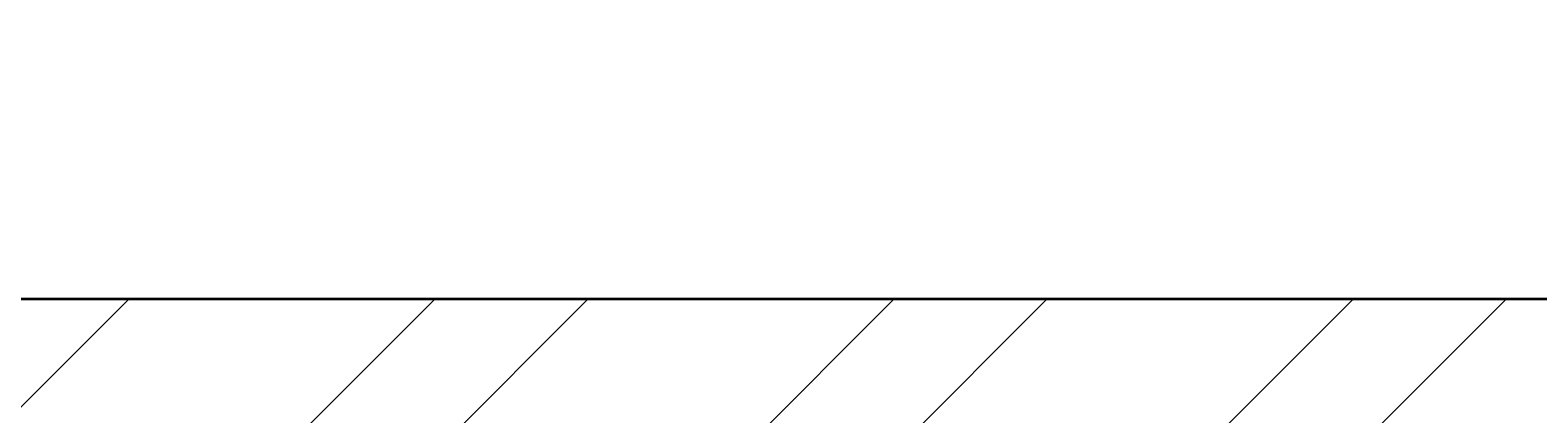
# Model space of a CAD drawing. Units: inches. Extents: x 1962 to 2771, y 1245 to 2660.
# Tile 41 of 114: x 2116 to 2160, y 2030 to 2042. Entities that reach past the tile are written whole.
import ezdxf

# ---------------------------------------------------------------- set-up
doc = ezdxf.new("R2010")
doc.units = ezdxf.units.IN
for name, color, linetype, lineweight in [('A-ANNO-DIMS', 2, 'Continuous', 18), ('A-WALL', 7, 'Continuous', 35), ('A-WALL-PATT', 252, 'Continuous', 13)]:
    doc.layers.add(name, color=color, linetype=linetype, lineweight=lineweight)
doc.styles.get("Standard").update_dxf_attribs({"font": 'arial.ttf'})
doc.dimstyles.get("Standard").update_dxf_attribs({"dimtxt": 0.18, "dimasz": 0.18, "dimexe": 0.18, "dimexo": 0.0625, "dimgap": 0.09, "dimtad": 0, "dimtih": 1, "dimtoh": 1, "dimdec": 4, "dimzin": 0, "dimdsep": 46, "dimtxsty": 'Standard', "dimcen": 0.09, "dimadec": 0, "dimazin": 0, "dimtfac": 1, "dimtdec": 4, "dimtofl": 0, "dimtmove": 0, "dimatfit": 3, "dimfxl": 1, "dimtolj": 1, "dimtzin": 0, "dimarcsym": 0})

# ---------------------------------------------------------------- blocks, each defined once
blk = doc.blocks.new('*D40')
at = {"layer": 'A-ANNO-DIMS', "color": 0, "lineweight": -2, "transparency": 16777216}
for p, q in [((2072.02, 2033.906), (2072.02, 2583.474)), ((2072.2, 2583.294), (2366.02, 2583.294)), ((2660.627, 2583.294), (2366.808, 2583.294)), ((2660.807, 2524.406), (2660.807, 2583.474))]:
    blk.add_line(p, q, dxfattribs=at)
at = {"layer": 'A-ANNO-DIMS', "color": 0, "transparency": 16777216}
for points in [[(2072.2, 2583.324), (2072.2, 2583.264), (2072.02, 2583.294)], [(2660.627, 2583.324), (2660.627, 2583.264), (2660.807, 2583.294)]]:
    blk.add_solid(points, dxfattribs=at)
at = {"layer": 'Defpoints', "color": 0, "transparency": 16777216}
for p in [(2660.807, 2583.294), (2660.807, 2524.344), (2072.02, 2033.844)]:
    blk.add_point(p, dxfattribs=at)
at = {"layer": 'A-ANNO-DIMS', "color": 0, "transparency": 16777216, "insert": (2366.414, 2583.294), "char_height": 0.18, "attachment_point": 5}
blk.add_mtext('\\A1;588.8', dxfattribs=at)

msp = doc.modelspace()

# ---------------------------------------------------------------- hatches: boundary and pattern name
at = {"layer": 'A-WALL-PATT'}
h = msp.add_hatch(dxfattribs=at)
h.set_pattern_fill('ANSI32', color=256)
h.paths.add_polyline_path([(2090.8074, 2467.3437), (2141.6481, 2467.3437), (2141.6481, 2469.5937), (2141.6481, 2471.8437), (2086.3074, 2471.8437), (2086.3074, 2422.5333), (2090.8074, 2422.5333)])
h.paths.add_polyline_path([(2282.7664, 2471.8437), (2204.8982, 2471.8437), (2204.8982, 2467.3437), (2234.8074, 2467.3437), (2234.8074, 2311.3437), (2228.7492, 2311.3437), (2228.7492, 2306.8437), (2234.8074, 2306.8437), (2331.9227, 2306.8437), (2331.9227, 2309.0937), (2331.9227, 2311.3437), (2239.3074, 2311.3437), (2239.3074, 2467.3437), (2282.7664, 2467.3437), (2282.7664, 2469.5937)])
h.paths.add_polyline_path([(2471.4531, 2519.8437), (2552.011, 2519.8437), (2564.3996, 2519.8437), (2564.3996, 2511.1389), (2568.8996, 2511.1389), (2568.8996, 2524.3437), (2466.9531, 2524.3437), (2466.9531, 2471.8437), (2450.0749, 2471.8437), (2446.4672, 2471.8437), (2446.4672, 2467.3437), (2450.0749, 2467.3437), (2475.9988, 2467.3437), (2475.9988, 2469.5937), (2475.9988, 2471.8437), (2471.4531, 2471.8437)])
h.paths.add_polyline_path([(2575.2231, 2469.5937), (2575.2231, 2471.8437), (2568.8996, 2471.8437), (2568.8996, 2487.1389), (2564.3996, 2487.1389), (2564.3996, 2471.8437), (2556.511, 2471.8437), (2499.2904, 2471.8437), (2499.2904, 2467.3437), (2507.8074, 2467.3437), (2507.8074, 2311.3437), (2414.863, 2311.3437), (2414.863, 2306.8437), (2512.3074, 2306.8437), (2517.0114, 2306.8437), (2517.0114, 2309.0937), (2517.0114, 2311.3437), (2512.3074, 2311.3437), (2512.3074, 2467.3437), (2575.2231, 2467.3437)])
h.paths.add_polyline_path([(2660.8074, 2471.8437), (2600.9602, 2471.8437), (2600.9602, 2467.3437), (2656.3074, 2467.3437), (2656.3074, 2432.5704), (2660.8074, 2432.5704)])
h.paths.add_polyline_path([(2660.8074, 2372.5704), (2656.3074, 2372.5704), (2656.3074, 2311.3437), (2600.276, 2311.3437), (2600.276, 2309.0937), (2600.276, 2306.8437), (2656.3074, 2306.8437), (2656.3074, 2296.2593), (2660.8074, 2296.2593)])
h.paths.add_polyline_path([(2572.3074, 2306.8437), (2577.1385, 2306.8437), (2577.1385, 2311.3437), (2551.082, 2311.3437), (2551.082, 2306.8437), (2567.8074, 2306.8437), (2567.8074, 2258.8437), (2540.0574, 2258.8437), (2540.0574, 2256.5937), (2540.0574, 2254.3437), (2567.8074, 2254.3437), (2656.3074, 2254.3437), (2656.3074, 2236.9085), (2660.8074, 2236.9085), (2660.8074, 2272.2593), (2656.3074, 2272.2593), (2656.3074, 2258.8437), (2572.3074, 2258.8437)])
h.paths.add_polyline_path([(2512.3074, 2254.3437), (2518.8716, 2254.3437), (2518.8716, 2256.5937), (2518.8716, 2258.8437), (2507.8074, 2258.8437), (2507.8074, 2177.8437), (2567.8074, 2177.8437), (2567.8074, 2172.9628), (2572.3074, 2172.9628), (2572.3074, 2177.8437), (2656.3074, 2177.8437), (2656.3074, 2166.4846), (2660.8074, 2166.4846), (2660.8074, 2200.9085), (2656.3074, 2200.9085), (2656.3074, 2182.3437), (2512.3074, 2182.3437)])
h.paths.add_polyline_path([(2656.3074, 2129.8437), (2572.3074, 2129.8437), (2572.3074, 2150.3044), (2570.0574, 2150.3044), (2567.8074, 2150.3044), (2567.8074, 2129.8437), (2507.8074, 2129.8437), (2507.8074, 2116.3027), (2510.0574, 2116.3027), (2512.3074, 2116.3027), (2512.3074, 2125.3437), (2567.8074, 2125.3437), (2572.3074, 2125.3437), (2656.3074, 2125.3437)])
h.paths.add_polyline_path([(2090.8074, 2362.5333), (2086.3074, 2362.5333), (2086.3074, 2298.6242), (2090.8074, 2298.6242), (2090.8074, 2306.8437), (2174.8074, 2306.8437), (2174.8074, 2286.4178), (2179.3074, 2286.4178), (2179.3074, 2306.8437), (2192.8641, 2306.8437), (2192.8641, 2309.0937), (2192.8641, 2311.3437), (2090.8074, 2311.3437)])
h.paths.add_polyline_path([(2209.156, 2258.8437), (2179.3074, 2258.8437), (2179.3074, 2263.2236), (2177.0574, 2263.2236), (2174.8074, 2263.2236), (2174.8074, 2258.8437), (2090.8074, 2258.8437), (2090.8074, 2274.6242), (2086.3074, 2274.6242), (2086.3074, 2238.2967), (2088.5574, 2238.2967), (2090.8074, 2238.2967), (2090.8074, 2254.3437), (2209.156, 2254.3437)])
h.paths.add_polyline_path([(2090.8074, 2177.8437), (2234.8074, 2177.8437), (2234.8074, 2173.1428), (2239.3074, 2173.1428), (2239.3074, 2258.8437), (2230.8442, 2258.8437), (2230.8442, 2256.5937), (2230.8442, 2254.3437), (2234.8074, 2254.3437), (2234.8074, 2182.3437), (2090.8074, 2182.3437), (2090.8074, 2202.2967), (2086.3074, 2202.2967), (2086.3074, 2140.0389), (2090.8074, 2140.0389)])
h.paths.add_polyline_path([(2090.8074, 2080.0389), (2086.3074, 2080.0389), (2086.3074, 2033.8437), (2090.8074, 2033.8437)], flags=17)
h.paths.add_polyline_path([(2244.9405, 2033.8437), (2239.3074, 2033.8437), (2239.3074, 2142.0665), (2237.2592, 2142.0665), (2234.8074, 2142.0665), (2234.8074, 2033.8437), (2090.8074, 2033.8437), (2076.5204, 2033.8437), (2072.0204, 2033.8437), (2072.0204, 2000.4493), (2076.5204, 2000.4493), (2076.5204, 2029.3437), (2090.8074, 2029.3437), (2244.9405, 2029.3437), (2244.9405, 2031.5937)])
h.paths.add_polyline_path([(2234.8074, 1933.3437), (2076.5204, 1933.3437), (2076.5204, 1952.4493), (2074.2704, 1952.4493), (2072.0204, 1952.4493), (2072.0204, 1933.3437), (2072.0204, 1928.8437), (2234.8074, 1928.8437)])
h.paths.add_polyline_path([(2090.8074, 1928.8437), (2086.3074, 1928.8437), (2086.3074, 1906.5013), (2090.8074, 1906.5013)])
h.paths.add_polyline_path([(2090.8074, 1846.5013), (2086.3074, 1846.5013), (2086.3074, 1769.9917), (2088.5574, 1769.9917), (2090.8074, 1769.9917), (2090.8074, 1780.3437), (2234.8074, 1780.3437), (2234.8074, 1708.3437), (2230.3764, 1708.3437), (2230.3764, 1703.8437), (2239.3074, 1703.8437), (2239.3074, 1792.6669), (2237.0574, 1792.6669), (2234.8074, 1792.6669), (2234.8074, 1784.8437), (2090.8074, 1784.8437)])
h.paths.add_polyline_path([(2239.3074, 1928.8437), (2244.9405, 1928.8437), (2244.9405, 1931.0937), (2244.9405, 1933.3437), (2234.8074, 1933.3437), (2234.8074, 1928.8437), (2234.8074, 1825.5949), (2239.3074, 1825.5949)])
h.paths.add_polyline_path([(2148.0425, 1649.0937), (2148.0425, 1651.3437), (2090.8074, 1651.3437), (2090.8074, 1646.8437), (2148.0425, 1646.8437)], flags=0)
h.paths.add_polyline_path([(2207.5601, 1708.3437), (2090.8074, 1708.3437), (2090.8074, 1703.8437), (2174.8074, 1703.8437), (2174.8074, 1651.3437), (2170.4457, 1651.3437), (2170.4457, 1646.8437), (2195.9924, 1646.8437), (2195.9924, 1649.0937), (2195.9924, 1651.3437), (2179.3074, 1651.3437), (2179.3074, 1703.8437), (2207.5601, 1703.8437), (2207.5601, 1706.0937)])
h.paths.add_polyline_path([(2090.8074, 1733.9917), (2086.3074, 1733.9917), (2086.3074, 1696.1032), (2088.5574, 1696.1032), (2090.8074, 1696.1032)])
h.paths.add_polyline_path([(2090.8074, 1672.1032), (2086.3074, 1672.1032), (2086.3074, 1600.3335), (2090.8074, 1600.3335)])
h.paths.add_polyline_path([(2090.8074, 1540.3335), (2086.3074, 1540.3335), (2086.3074, 1486.3437), (2139.6766, 1486.3437), (2139.6766, 1490.8437), (2090.8074, 1490.8437)])
h.paths.add_polyline_path([(2302.3876, 1490.8437), (2239.3074, 1490.8437), (2239.3074, 1646.8437), (2335.9994, 1646.8437), (2335.9994, 1651.3437), (2229.884, 1651.3437), (2229.884, 1646.8437), (2234.8074, 1646.8437), (2234.8074, 1490.8437), (2202.7103, 1490.8437), (2202.7103, 1488.5937), (2202.7103, 1486.3437), (2275.0699, 1486.3437), (2275.0699, 1475.772), (2279.5699, 1475.772), (2279.5699, 1486.3437), (2302.3876, 1486.3437)])
h.paths.add_polyline_path([(2279.5699, 1451.772), (2275.0699, 1451.772), (2275.0699, 1438.3437), (2174.8074, 1438.3437), (2174.8074, 1486.3437), (2179.7922, 1486.3437), (2179.7922, 1490.8437), (2163.3585, 1490.8437), (2163.3585, 1488.5937), (2163.3585, 1486.3437), (2170.3074, 1486.3437), (2170.3074, 1433.8437), (2279.5699, 1433.8437)])
h.paths.add_polyline_path([(2427.2363, 1490.8437), (2375.8074, 1490.8437), (2375.8074, 1646.8437), (2381.6401, 1646.8437), (2381.6401, 1651.3437), (2365.887, 1651.3437), (2365.887, 1649.0937), (2365.887, 1646.8437), (2371.3074, 1646.8437), (2371.3074, 1490.8437), (2327.5627, 1490.8437), (2327.5627, 1488.5937), (2327.5627, 1486.3437), (2371.3074, 1486.3437), (2371.3074, 1433.8437), (2375.8074, 1433.8437), (2375.8074, 1486.3437), (2427.2363, 1486.3437)])
h.paths.add_polyline_path([(2512.3074, 1646.8437), (2519.4351, 1646.8437), (2519.4351, 1649.0937), (2519.4351, 1651.3437), (2507.8074, 1651.3437), (2416.0063, 1651.3437), (2416.0063, 1649.0937), (2416.0063, 1646.8437), (2507.8074, 1646.8437), (2507.8074, 1490.8437), (2497.0532, 1490.8437), (2497.0532, 1488.5937), (2497.0532, 1486.3437), (2574.9344, 1486.3437), (2574.9344, 1476.0181), (2579.4344, 1476.0181), (2579.4344, 1486.3437), (2584.4872, 1486.3437), (2584.3074, 1490.8437), (2512.3074, 1490.8437)])
h.paths.add_polyline_path([(2470.5091, 1486.3437), (2473.9767, 1486.3437), (2473.9767, 1490.8437), (2449.6605, 1490.8437), (2449.6605, 1488.5937), (2449.6605, 1486.3437), (2466.0091, 1486.3437), (2466.0091, 1433.8437), (2470.5091, 1433.8437), (2579.4344, 1433.8437), (2579.4344, 1452.0181), (2574.9344, 1452.0181), (2574.9344, 1438.3437), (2554.5091, 1438.3437), (2470.5091, 1438.3437)])
h.paths.add_polyline_path([(2656.3074, 1490.8437), (2611.86, 1490.8437), (2611.86, 1486.3437), (2656.3074, 1486.3437)])
h.paths.add_polyline_path([(2660.8074, 1532.7007), (2658.5574, 1532.7007), (2656.3074, 1532.7007), (2656.3074, 1486.3437), (2660.8074, 1486.3437)])
h.paths.add_polyline_path([(2660.8074, 1664.9663), (2656.3074, 1664.9663), (2656.3074, 1651.3437), (2602.2313, 1651.3437), (2602.2313, 1646.8437), (2656.3074, 1646.8437), (2656.3074, 1592.7007), (2660.8074, 1592.7007)])
h.paths.add_polyline_path([(2660.8074, 1724.5221), (2656.3074, 1724.5221), (2656.3074, 1703.8437), (2542.4725, 1703.8437), (2542.4725, 1699.3437), (2567.8074, 1699.3437), (2567.8074, 1651.3437), (2552.7766, 1651.3437), (2552.7766, 1649.0937), (2552.7766, 1646.8437), (2577.2878, 1646.8437), (2577.2878, 1649.0937), (2577.2878, 1651.3437), (2572.3074, 1651.3437), (2572.3074, 1699.3437), (2656.3074, 1699.3437), (2656.3074, 1688.9663), (2660.8074, 1688.9663)])
h.paths.add_polyline_path([(2660.8074, 1880.6524), (2656.3074, 1880.6524), (2656.3074, 1832.8437), (2512.3074, 1832.8437), (2512.3074, 1837.8959), (2507.8074, 1837.8959), (2507.8074, 1828.3437), (2567.8074, 1828.3437), (2567.8074, 1804.3437), (2572.3074, 1804.3437), (2572.3074, 1828.3437), (2656.3074, 1828.3437), (2656.3074, 1818.6778), (2660.8074, 1818.6778)])
h.paths.add_polyline_path([(2660.8074, 1794.6778), (2656.3074, 1794.6778), (2656.3074, 1780.3437), (2572.3074, 1780.3437), (2572.3074, 1783.0303), (2570.0574, 1783.0303), (2567.8074, 1783.0303), (2567.8074, 1780.3437), (2507.8074, 1780.3437), (2507.8074, 1699.3437), (2517.8858, 1699.3437), (2517.8858, 1701.5937), (2517.8858, 1703.8437), (2512.3074, 1703.8437), (2512.3074, 1775.8437), (2656.3074, 1775.8437), (2656.3074, 1760.5221), (2660.8074, 1760.5221)])
h.paths.add_polyline_path([(2660.8074, 1981.3437), (2660.8074, 2020.2808), (2658.5574, 2020.2808), (2656.3074, 2020.2808), (2656.3074, 1981.3437), (2512.3074, 1981.3437), (2512.3074, 2086.6996), (2507.8074, 2086.6996), (2507.8074, 1981.3437), (2375.8074, 1981.3437), (2375.8074, 1986.8505), (2373.5574, 1986.8505), (2371.3074, 1986.8505), (2371.3074, 1973.2607), (2375.8074, 1973.2607), (2375.8074, 1976.8437), (2507.8074, 1976.8437), (2507.8074, 1865.4281), (2510.0574, 1865.4281), (2512.3074, 1865.4281), (2512.3074, 1976.8437), (2660.8074, 1976.8437)])
h.paths.add_polyline_path([(2375.8074, 1940.297), (2373.5574, 1940.297), (2371.3074, 1940.297), (2371.3074, 1933.3437), (2278.4434, 1933.3437), (2278.4434, 1928.8437), (2371.3074, 1928.8437), (2371.3074, 1651.3437), (2375.8074, 1651.3437)])
h.paths.add_polyline_path([(2660.8074, 1976.8437), (2656.3074, 1976.8437), (2656.3074, 1940.6524), (2660.8074, 1940.6524)], flags=17)
h.paths.add_polyline_path([(2660.8074, 2142.4846), (2656.3074, 2142.4846), (2656.3074, 2080.2808), (2660.8074, 2080.2808)])
h.paths.add_polyline_path([(2381.4189, 2311.3437), (2375.8074, 2311.3437), (2375.8074, 2467.3437), (2424.7242, 2467.3437), (2424.7242, 2469.5937), (2424.7242, 2471.8437), (2375.8074, 2471.8437), (2375.8074, 2524.3437), (2371.3074, 2524.3437), (2371.3074, 2471.8437), (2307.2097, 2471.8437), (2307.2097, 2467.3437), (2371.3074, 2467.3437), (2371.3074, 2311.3437), (2366.8901, 2311.3437), (2366.8901, 2306.8437), (2371.3074, 2306.8437), (2371.3074, 2033.8437), (2279.6589, 2033.8437), (2279.6589, 2029.3437), (2371.3074, 2029.3437), (2371.3074, 2014.2598), (2375.8074, 2014.2598), (2375.8074, 2306.8437), (2381.4189, 2306.8437)])
h.paths.add_polyline_path([(2263.3074, 2524.3437), (2170.3074, 2524.3437), (2170.3074, 2519.8437), (2170.3074, 2471.8437), (2165.0312, 2471.8437), (2165.0312, 2467.3437), (2179.6721, 2467.3437), (2179.6721, 2469.5161), (2179.6721, 2471.8437), (2174.8074, 2471.8437), (2174.8074, 2519.8437), (2258.8074, 2519.8437), (2258.8074, 2511.6436), (2263.3074, 2511.6436)])
h.paths.add_polyline_path([(2245.0232, 1361.4123), (2492.9468, 1361.4123), (2492.9468, 1398.505), (2245.0232, 1398.505)], flags=9)
h.paths.add_polyline_path([(2388.1434, 2086.6936), (2425.0704, 2086.6936), (2425.0704, 2105.3509), (2388.1434, 2105.3509)], flags=9)
h.paths.add_polyline_path([(2404.922, 2242.6744), (2445.7337, 2242.6744), (2445.7337, 2261.3318), (2404.922, 2261.3318)], flags=9)
h.paths.add_polyline_path([(2269.4107, 2156.7935), (2306.3378, 2156.7935), (2306.3378, 2175.4508), (2269.4107, 2175.4508)], flags=9)
h.paths.add_polyline_path([(2269.3277, 2233.4343), (2306.2547, 2233.4343), (2306.2547, 2252.0917), (2269.3277, 2252.0917)], flags=9)
h.paths.add_polyline_path([(2431.6052, 2320.6922), (2470.4456, 2320.6922), (2470.4456, 2339.3495), (2431.6052, 2339.3495)], flags=25)
h.paths.add_polyline_path([(2249.6902, 2315.7608), (2288.5306, 2315.7608), (2288.5306, 2334.4182), (2249.6902, 2334.4182)], flags=25)
h.paths.add_polyline_path([(2096.9301, 2314.3181), (2135.7704, 2314.3181), (2135.7704, 2332.9755), (2096.9301, 2332.9755)], flags=25)
h.paths.add_polyline_path([(2134.3475, 2285.7089), (2161.4655, 2285.7089), (2161.4655, 2304.3662), (2134.3475, 2304.3662)], flags=9)
h.paths.add_polyline_path([(2126.5155, 2209.4076), (2159.9227, 2209.4076), (2159.9227, 2228.065), (2126.5155, 2228.065)], flags=25)
h.paths.add_polyline_path([(2110.5753, 2141.5299), (2149.4157, 2141.5299), (2149.4157, 2160.1872), (2110.5753, 2160.1872)], flags=25)
h.paths.add_polyline_path([(2249.8618, 1968.3317), (2286.3966, 1968.3317), (2286.3966, 1986.989), (2249.8618, 1986.989)], flags=9)
h.paths.add_polyline_path([(2395.9507, 1777.0051), (2436.7624, 1777.0051), (2436.7624, 1795.6625), (2395.9507, 1795.6625)], flags=9)
h.paths.add_polyline_path([(2398.5259, 1888.5651), (2435.0062, 1888.5651), (2435.0062, 1907.2224), (2398.5259, 1907.2224)], flags=25)
h.paths.add_polyline_path([(2259.3506, 1728.3559), (2296.2776, 1728.3559), (2296.2776, 1747.0132), (2259.3506, 1747.0132)], flags=9)
h.paths.add_polyline_path([(2271.3698, 1845.268), (2308.2968, 1845.268), (2308.2968, 1863.9253), (2271.3698, 1863.9253)], flags=9)
h.paths.add_polyline_path([(2120.9355, 1786.3027), (2159.7759, 1786.3027), (2159.7759, 1804.9601), (2120.9355, 1804.9601)], flags=25)
h.paths.add_polyline_path([(2121.3164, 1732.1043), (2154.7236, 1732.1043), (2154.7236, 1750.7616), (2121.3164, 1750.7616)], flags=25)
h.paths.add_polyline_path([(2118.3706, 1678.8997), (2147.5282, 1678.8997), (2147.5282, 1697.557), (2118.3706, 1697.557)], flags=25)
h.paths.add_polyline_path([(2385.9227, 1493.557), (2424.763, 1493.557), (2424.763, 1512.2143), (2385.9227, 1512.2143)], flags=25)
h.paths.add_polyline_path([(2248.7058, 1500.0256), (2287.5462, 1500.0256), (2287.5462, 1518.6829), (2248.7058, 1518.6829)], flags=25)
h.paths.add_polyline_path([(2104.1669, 1617.3771), (2143.0073, 1617.3771), (2143.0073, 1636.0344), (2104.1669, 1636.0344)], flags=9)
h.paths.add_polyline_path([(2096.0714, 1447.8824), (2137.3845, 1447.8824), (2137.3845, 1458.1859), (2096.0714, 1458.1859)], flags=9)
h.paths.add_polyline_path([(2180.6114, 1440.325), (2209.7689, 1440.325), (2209.7689, 1458.9823), (2180.6114, 1458.9823)], flags=25)
h.paths.add_polyline_path([(2316.1698, 1447.9637), (2357.4829, 1447.9637), (2357.4829, 1458.2673), (2316.1698, 1458.2673)], flags=9)
h.paths.add_polyline_path([(2397.6187, 1447.9637), (2438.9318, 1447.9637), (2438.9318, 1458.2673), (2397.6187, 1458.2673)], flags=9)
h.paths.add_polyline_path([(2473.0778, 1439.5953), (2502.2354, 1439.5953), (2502.2354, 1458.2527), (2473.0778, 1458.2527)], flags=25)
h.paths.add_polyline_path([(2589.7027, 1447.8819), (2631.0158, 1447.8819), (2631.0158, 1458.1855), (2589.7027, 1458.1855)], flags=9)
h.paths.add_polyline_path([(2522.4009, 1497.5285), (2561.2413, 1497.5285), (2561.2413, 1516.1859), (2522.4009, 1516.1859)], flags=25)
h.paths.add_polyline_path([(2579.6565, 1671.3482), (2608.8141, 1671.3482), (2608.8141, 1690.0056), (2579.6565, 1690.0056)], flags=25)
h.paths.add_polyline_path([(2544.7038, 1725.5064), (2578.1111, 1725.5064), (2578.1111, 1744.1637), (2544.7038, 1744.1637)], flags=25)
h.paths.add_polyline_path([(2578.1191, 1807.472), (2607.2766, 1807.472), (2607.2766, 1826.1293), (2578.1191, 1826.1293)], flags=25)
h.paths.add_polyline_path([(2595.0614, 1835.1839), (2633.9018, 1835.1839), (2633.9018, 1853.8413), (2595.0614, 1853.8413)], flags=25)
h.paths.add_polyline_path([(2567.0097, 2097.7035), (2605.8501, 2097.7035), (2605.8501, 2116.3609), (2567.0097, 2116.3609)], flags=9)
h.paths.add_polyline_path([(2586.644, 2134.6454), (2615.8015, 2134.6454), (2615.8015, 2153.3027), (2586.644, 2153.3027)], flags=9)
h.paths.add_polyline_path([(2544.6185, 2212.6783), (2578.0258, 2212.6783), (2578.0258, 2231.3356), (2544.6185, 2231.3356)], flags=25)
h.paths.add_polyline_path([(2577.0273, 2256.9023), (2606.1849, 2256.9023), (2606.1849, 2275.5597), (2577.0273, 2275.5597)], flags=24)
h.paths.add_polyline_path([(2605.2683, 2315.2821), (2644.1087, 2315.2821), (2644.1087, 2333.9395), (2605.2683, 2333.9395)], flags=25)
h.paths.add_polyline_path([(2583.1244, 2496.1815), (2624.4375, 2496.1815), (2624.4375, 2506.4851), (2583.1244, 2506.4851)], flags=9)
h.paths.add_polyline_path([(2474.761, 2497.0823), (2503.9185, 2497.0823), (2503.9185, 2515.7397), (2474.761, 2515.7397)], flags=25)
h.paths.add_polyline_path([(2387.5787, 2494.2563), (2428.902, 2494.2563), (2428.902, 2504.5598), (2387.5787, 2504.5598)], flags=9)
h.paths.add_polyline_path([(2300.1657, 2500.1564), (2341.4788, 2500.1564), (2341.4788, 2510.46), (2300.1657, 2510.46)], flags=25)
h.paths.add_polyline_path([(2176.8589, 2497.5843), (2206.0165, 2497.5843), (2206.0165, 2516.2416), (2176.8589, 2516.2416)], flags=25)
h.paths.add_polyline_path([(2097.4668, 2494.9762), (2138.7799, 2494.9762), (2138.7799, 2505.2798), (2097.4668, 2505.2798)], flags=9)

# ---------------------------------------------------------------- linework, layer by layer
at = {"layer": 'A-WALL'}
msp.add_line((2090.8074, 2033.8437), (2234.8074, 2033.8437), dxfattribs=at)

# ---------------------------------------------------------------- dimensions: what is measured, and where the dimension line sits
at = {"layer": 'A-ANNO-DIMS'}
dim = msp.add_linear_dim(base=(2660.8074, 2583.2937), p1=(2072.0204, 2033.8437), p2=(2660.8074, 2524.3437), dimstyle='Standard', override={"dimdec": 1, "dimlfac": 1, "dimrnd": 0, "dimzin": 0, "dimdsep": 46, "dimlunit": 2}, dxfattribs=at)
dim.commit()
dim.dimension.update_dxf_attribs({"geometry": '*D40', "text_midpoint": (2366.4139, 2583.2937)})

doc.saveas('drawing.dxf')
